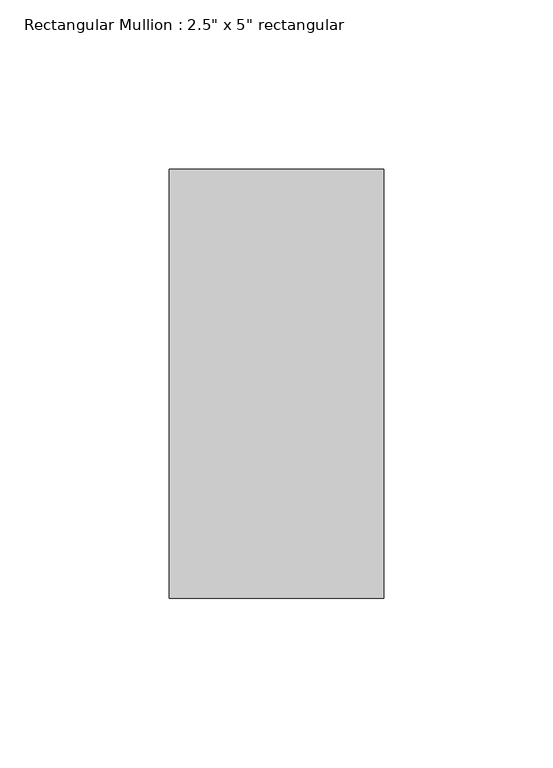
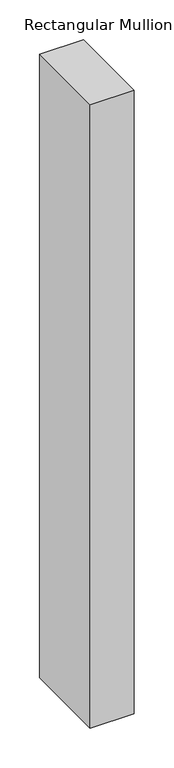
"""IFC4 building model written with IfcOpenShell, lengths in millimetres: member geometry."""

from ifc_helpers import new_model, si_unit, frame, origin, place, context, project, spatial, polyline, outline, extrude, source, transform, mapped, element, save


def member_3b6b664d(model_context):
    return source(origin(), model_context, "Body", "SweptSolid", [
        extrude(outline(polyline([(0.0, 63.5), (0.0, -63.5), (-63.5, -63.5), (-63.5, 63.5), (0.0, 63.5)])), frame((0.0, 0.0, -954.6166668), z_axis=(0.0, 0.0, 1.0), x_axis=(1.0, 0.0, 0.0)), (0.0, 0.0, 1.0), 954.6166668),
    ])


if __name__ == "__main__":
    model = new_model("IFC4")
    model_context = context("Model", 3, world=origin())
    ifc_project = project(units=[si_unit("LENGTHUNIT", "METRE", prefix="MILLI")], contexts=[model_context])
    site = spatial("IfcSite", under=ifc_project)
    building = spatial("IfcBuilding", under=site)
    placement = place(None, origin())
    member_shape = member_3b6b664d(model_context)
    element("IfcMember", 1, ObjectType="Rectangular Mullion : 2.5\" x 5\" rectangular", at=placement, inside=building, context=model_context, shape_type="MappedRepresentation", body=[
        mapped(member_shape, transform((0.0, 0.0, 0.0), x_axis=(1.0, 0.0, 0.0), y_axis=(0.0, 1.0, 0.0), z_axis=(0.0, 0.0, 1.0))),
    ])
    save(model, "model.ifc")

# Revit data of these elements
# Type "Rectangular Mullion : 2.5\" x 5\" rectangular"
#   built-in parameter 1007304 = 0.416667 (stored number, unit not read)
#   built-in parameter 1007301 = 0.104167 (stored number, unit not read)
#   built-in parameter 1007300 = 0.104167 (stored number, unit not read)
# Element 1 (IfcMember, "Rectangular Mullion : 2.5\" x 5\" rectangular")
#   Materials on its faces: "Aluminum"
# Materials
#   "Aluminum": class "Metal", colour RGB 247 247 247, transparency 0, Description = "Aluminum 6061", Cost = 0
